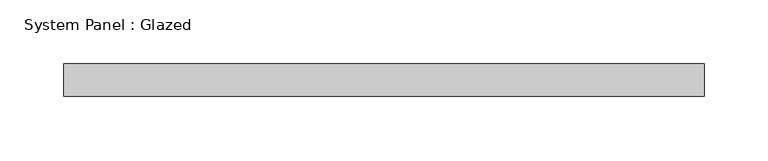
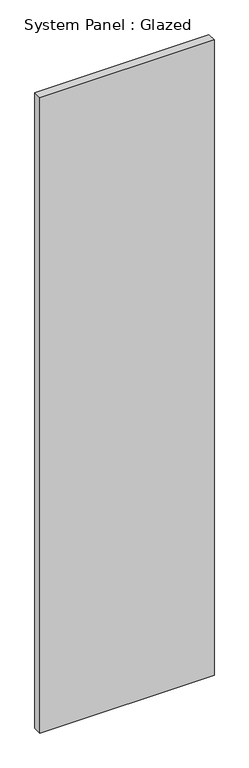
"""IFC4 building model written with IfcOpenShell, lengths in millimetres: plate geometry, System Panel : Glazed."""

from ifc_helpers import new_model, si_unit, origin, origin_with_axes, place, context, project, spatial, polyline, outline, extrude, source, transform, mapped, element, save


def system_panel_glazed_83f38206(model_context):
    return source(origin(), model_context, "Body", "SweptSolid", [
        extrude(outline(polyline([(250.825, 19.05), (-250.825, 19.05), (-250.825, 44.45), (250.825, 44.45), (250.825, 19.05)])), origin_with_axes(), (0.0, 0.0, 1.0), 1936.6147749),
    ])


if __name__ == "__main__":
    model = new_model("IFC4")
    model_context = context("Model", 3, world=origin())
    ifc_project = project(units=[si_unit("LENGTHUNIT", "METRE", prefix="MILLI")], contexts=[model_context])
    site = spatial("IfcSite", under=ifc_project)
    building = spatial("IfcBuilding", under=site)
    placement = place(None, origin())
    system_panel_glazed_shape = system_panel_glazed_83f38206(model_context)
    element("IfcPlate", 1, ObjectType="System Panel : Glazed", at=placement, inside=building, context=model_context, shape_type="MappedRepresentation", body=[
        mapped(system_panel_glazed_shape, transform((0.0, 0.0, 0.0), x_axis=(1.0, 0.0, 0.0), y_axis=(0.0, 1.0, 0.0), z_axis=(0.0, 0.0, 1.0))),
    ])
    save(model, "model.ifc")

# Revit data of these elements
# Type "System Panel : Glazed"
#   Construction Type Id = "GSP4R"
#   Analytic Construction = "1/8 in Pilkington single glazing"
#   Visual Light Transmittance = 0.9
#   Solar Heat Gain Coefficient = 0.86
#   Heat Transfer Coefficient (U) = 1.18115 BTU/(h·ft²·°F)
#   Define Thermal Properties by = 1
# Element 1 (IfcPlate, "System Panel : Glazed")
#   Materials on its faces: "Glass"
# Materials
#   "Glass": class "Glass", colour RGB 0 128 192, transparency 0.75, Description = "Soda Lime Glass", Cost = 0
